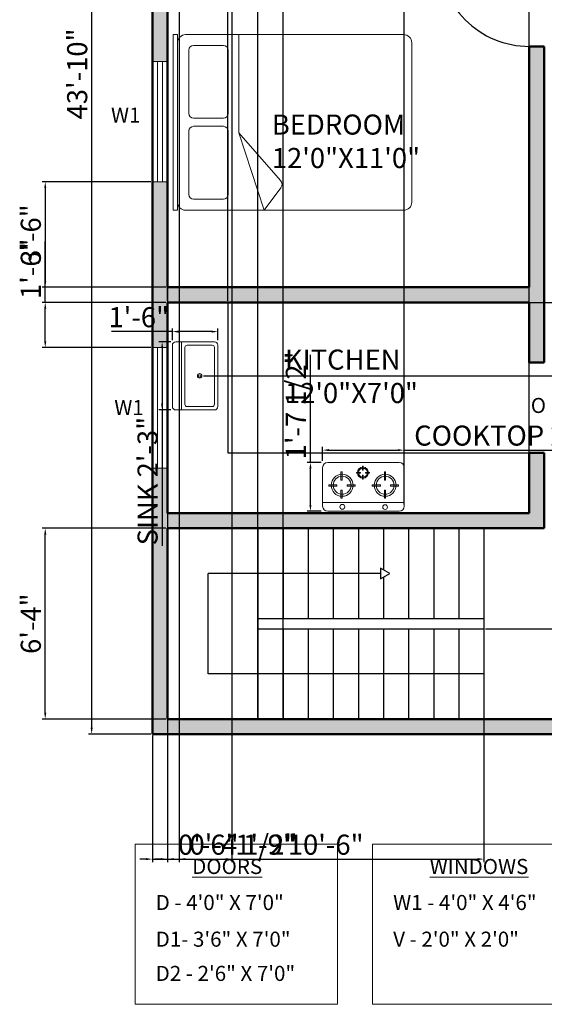
# Model space of a CAD drawing. Units: inches. Extents: x 3655 to 4051, y 2160 to 2854.
# Tile 1 of 3: x 3655 to 3863, y 2160 to 2552. Entities that reach past the tile are written whole.
import ezdxf

# ---------------------------------------------------------------- set-up
doc = ezdxf.new("R2010")
doc.units = ezdxf.units.IN
for name, color, linetype, lineweight in [('A-ANNO-DIMS', 2, 'Continuous', 18), ('A-ANNO-SCHD', 7, 'Continuous', 18), ('A-ANNO-TEXT', 7, 'Continuous', 18), ('A-AREA-IDEN', 7, 'Continuous', 25), ('A-DOOR', 3, 'Continuous', 25), ('A-EQPM', 9, 'Continuous', 18), ('A-FLOR-CASE', 8, 'Continuous', 25), ('A-FLOR-FIXT', 9, 'Continuous', 18), ('A-FLOR-STRS', 7, 'Continuous', 25), ('A-FURN', 8, 'Continuous', 18), ('A-GLAZ', 4, 'Continuous', 18), ('A-WALL', 7, 'Continuous', 50)]:
    doc.layers.add(name, color=color, linetype=linetype, lineweight=lineweight)
doc.layers.add('A-WALL-PATT', color=244, linetype='Continuous', lineweight=13, true_color=0x991b1e)
doc.styles.add('ATTR', font='romans.shx', dxfattribs={"width": 0.8, "height": 1.075})
doc.styles.get("Standard").update_dxf_attribs({"font": 'arial.ttf'})
doc.dimstyles.new('ISO-25', dxfattribs={"dimtxt": 8, "dimasz": 2.5, "dimexe": 1.25, "dimexo": 0.625, "dimtad": 1, "dimdec": 1, "dimlunit": 3, "dimtxsty": 'Standard', "dimcen": 2.5, "dimadec": 0, "dimazin": 0, "dimtfac": 1, "dimtdec": 1, "dimtmove": 0, "dimatfit": 3, "dimfxl": 1, "dimarcsym": 0})

# ---------------------------------------------------------------- blocks, each defined once
blk = doc.blocks.new('*U4')
for p, q in [((0, 0), (0, 6)), ((36, 0), (36, 6))]:
    blk.add_line(p, q)
blk.add_lwpolyline([(0, 0), (0, -36), (1.75, -36), (1.75, 0)], close=True)
blk.add_arc((0, 0), 36, 270, 0)
blk = doc.blocks.new('A$C164346CA')
for p, q in [((0, 2.035), (0, 2)), ((1.5, 2.035), (0, 2.035)), ((1.5, 2), (1.5, 2.035)), ((1.5, 2), (0, 2)), ((0, 1.93), (0, 0.07)), ((0.0919, 1.8624), (0.0919, 1.6069)), ((0.6731, 1.9024), (0.1319, 1.9024)), ((0.7131, 1.6069), (0.7131, 1.8624)), ((0.7828, 1.8624), (0.7828, 1.6069)), ((1.364, 1.9024), (0.8228, 1.9024)), ((1.404, 1.6069), (1.404, 1.8624)), ((1.5, 0.07), (1.5, 1.93)), ((0.1319, 1.5669), (0.6731, 1.5669)), ((0.8228, 1.5669), (1.364, 1.5669)), ((0.8395, 1.4761), (0, 1.4761)), ((0.8395, 1.4761), (1.2448, 1.12)), ((1.5, 1.2611), (0.8395, 1.4761)), ((1.3077, 1.1175), (1.5, 1.2611)), ((0.07, 0), (1.43, 0))]:
    blk.add_line(p, q)
for centre, radius, start, end in [((0.07, 1.93), 0.07, 90, 180), ((1.43, 1.93), 0.07, 0, 90), ((0.1319, 1.8624), 0.04, 90, 180), ((0.6731, 1.8624), 0.04, 0, 90), ((0.8228, 1.8624), 0.04, 90, 180), ((1.364, 1.8624), 0.04, 0, 90), ((0.1319, 1.6069), 0.04, 180, 270), ((0.6731, 1.6069), 0.04, 270, 0), ((0.8228, 1.6069), 0.04, 180, 270), ((1.364, 1.6069), 0.04, 270, 0), ((1.2778, 1.1575), 0.05, 228.69584, 306.75789), ((0.07, 0.07), 0.07, 180, 270), ((1.43, 0.07), 0.07, 270, 0)]:
    blk.add_arc(centre, radius, start, end)
blk = doc.blocks.new('A$C2A3C6842')
for p, q in [((0, 45), (0, 387)), ((45, 432), (675, 432)), ((351.6, 363.3), (351.6, 398.9)), ((351.6, 398.9), (357.3, 398.9)), ((357.3, 363.3), (351.6, 363.3)), ((357.3, 398.9), (357.3, 363.3)), ((720, 387), (720, 45)), ((161.8, 346.9), (173.2, 346.9)), ((161.8, 275.6), (161.8, 346.9)), ((173.2, 275.6), (161.8, 275.6)), ((173.2, 346.9), (173.2, 275.6)), ((298.4, 341.9), (298.4, 336.2)), ((334, 341.9), (298.4, 341.9)), ((298.4, 336.2), (334, 336.2)), ((334, 336.2), (334, 341.9)), ((357.3, 318.8), (351.6, 318.8)), ((351.6, 318.8), (351.6, 283.1)), ((351.6, 283.1), (357.3, 283.1)), ((357.3, 283.1), (357.3, 318.8)), ((378.5, 336.2), (378.5, 341.9)), ((378.5, 341.9), (414.2, 341.9)), ((414.2, 336.2), (378.5, 336.2)), ((414.2, 341.9), (414.2, 336.2)), ((544.7, 346.9), (556.1, 346.9)), ((544.7, 275.6), (544.7, 346.9)), ((556.1, 275.6), (544.7, 275.6)), ((556.1, 346.9), (556.1, 275.6)), ((55.3, 232.9), (55.3, 221.5)), ((126.6, 232.9), (55.3, 232.9)), ((55.3, 221.5), (126.6, 221.5)), ((126.6, 221.5), (126.6, 232.9)), ((173.2, 186.6), (161.8, 186.6)), ((161.8, 186.6), (161.8, 115.3)), ((173.2, 115.3), (173.2, 186.6)), ((215.6, 221.5), (215.6, 232.9)), ((215.6, 232.9), (286.9, 232.9)), ((286.9, 221.5), (215.6, 221.5)), ((286.9, 232.9), (286.9, 221.5)), ((438.2, 232.9), (438.2, 221.5)), ((509.5, 232.9), (438.2, 232.9)), ((438.2, 221.5), (509.5, 221.5)), ((509.5, 221.5), (509.5, 232.9)), ((556.1, 186.6), (544.7, 186.6)), ((544.7, 186.6), (544.7, 115.3)), ((556.1, 115.3), (556.1, 186.6)), ((598.5, 232.9), (669.8, 232.9)), ((598.5, 221.5), (598.5, 232.9)), ((669.8, 221.5), (598.5, 221.5)), ((669.8, 232.9), (669.8, 221.5)), ((161.8, 115.3), (173.2, 115.3)), ((544.7, 115.3), (556.1, 115.3)), ((1.2, 76.7), (719.9, 76.7)), ((675, 0), (45, 0))]:
    blk.add_line(p, q)
at = {"extrusion": (0, -1e-16, -1)}
for centre, major_axis, start_param, end_param in [((45, 387), (31.8, 31.8), 3.926991, 5.497787), ((172.2, 229.8), (-97.3, 0.1), -0.001099, 6.282086), ((551.8, 229.8), (-97.3, 0.1), -0.001099, 6.282086), ((173.7, 39), (-14.8, 14.8), 5.497787, 11.780972)]:
    blk.add_ellipse(centre, major_axis=major_axis, ratio=1, start_param=start_param, end_param=end_param, dxfattribs=at)
at = {"extrusion": (-1e-16, -1e-16, -1)}
blk.add_ellipse((355.1, 340.4), major_axis=(48.7, 0.1), ratio=1, start_param=3.144125, end_param=9.42731, dxfattribs=at)
at = {"extrusion": (-1e-16, 0, -1)}
for centre, major_axis, start_param, end_param in [((355.1, 340.4), (-39.7, 0), -0.000334, 6.282851), ((45, 45), (-31.8, 31.8), 3.926991, 5.497787)]:
    blk.add_ellipse(centre, major_axis=major_axis, ratio=1, start_param=start_param, end_param=end_param, dxfattribs=at)
at = {"extrusion": (0, 1e-16, -1)}
blk.add_ellipse((675, 387), major_axis=(-31.8, 31.8), ratio=1, start_param=0.785398, end_param=2.356194, dxfattribs=at)
at = {"extrusion": (-1e-16, -4e-16, -1)}
for centre in [(172.2, 229.8), (551.8, 229.8)]:
    blk.add_ellipse(centre, major_axis=(-79.3, 0), ratio=1, start_param=-0.0002116186602152, end_param=6.282973688519371, dxfattribs=at)
at = {"extrusion": (2e-16, -2e-16, -1)}
blk.add_ellipse((551.4, 36.4), major_axis=(14.8, 14.8), ratio=1, start_param=3.926991, end_param=10.210176, dxfattribs=at)
at = {"extrusion": (-2e-16, 1e-16, -1)}
blk.add_ellipse((675, 45), major_axis=(31.8, 31.8), ratio=1, start_param=0.785398, end_param=2.356194, dxfattribs=at)
at = {"text_generation_flag": 4, "flags": 9}
for tag in ['XSIZE', 'YSIZE']:
    blk.add_attdef(tag, (361.3, 264.9), '', height=0.45, rotation=180, dxfattribs=at)
blk = doc.blocks.new("30'' Sink Single PV")
blk.add_line((-15, -3.999996), (15, -3.999996))
for points in [[(-13.5, 0), (13.5, 0)], [(-15, -18.499996), (-15, -1.5)], [(15, -1.5), (15, -18.499996)], [(-13.5, -17.499996), (-13.5, -6.499996)], [(-12.5, -5.499996), (12.5, -5.499996)], [(13.5, -6.499996), (13.5, -17.499996)], [(13.5, -19.999996), (-13.5, -19.999996)], [(12.5, -18.499996), (-12.5, -18.499996)]]:
    blk.add_lwpolyline(points)
for radius in [1, 0.5]:
    blk.add_circle((0, -11.999996), radius)
for centre, radius, start, end in [((-13.5, -1.5), 1.5, 90, 180), ((13.5, -1.5), 1.5, 0, 90), ((-12.5, -6.499996), 1, 90, 180), ((12.5, -6.499996), 1, 0, 90), ((-13.5, -18.499996), 1.5, 180, 270), ((-12.5, -17.499996), 1, 180, 270), ((12.5, -17.499996), 1, 270, 0), ((13.5, -18.499996), 1.5, 270, 0)]:
    blk.add_arc(centre, radius, start, end)
at = {"style": 'ATTR', "width": 0.8, "flags": 9}
blk.add_attdef('ESTCODE', (0, 0), '', height=0.006, dxfattribs=at)
blk = doc.blocks.new('*D13')
at = {"layer": 'A-ANNO-DIMS', "color": 0, "lineweight": -2, "transparency": 16777216}
for p, q in [((3706.78, 2793.69), (3682, 2793.69)), ((3683.25, 2791.19), (3683.25, 2270.19)), ((3706.78, 2267.69), (3682, 2267.69))]:
    blk.add_line(p, q, dxfattribs=at)
at = {"layer": 'A-ANNO-DIMS', "color": 0, "transparency": 16777216}
for points in [[(3682.83, 2791.19), (3683.66, 2791.19), (3683.25, 2793.69)], [(3682.83, 2270.19), (3683.66, 2270.19), (3683.25, 2267.69)]]:
    blk.add_solid(points, dxfattribs=at)
at = {"layer": 'Defpoints', "color": 0, "transparency": 16777216}
for p in [(3707.41, 2793.69), (3683.25, 2267.69), (3707.41, 2267.69)]:
    blk.add_point(p, dxfattribs=at)
at = {"layer": 'A-ANNO-DIMS', "color": 0, "transparency": 16777216, "insert": (3678.53, 2530.69), "char_height": 8, "attachment_point": 5, "rotation": 90}
blk.add_mtext('43\'-10"', dxfattribs=at)
blk = doc.blocks.new('WIN-W1-48IN')
for p, q in [((0, 0), (0, 6)), ((48, 4), (0, 4)), ((48, 0), (48, 6)), ((48, 2), (0, 2))]:
    blk.add_line(p, q)
blk = doc.blocks.new('*D20')
at = {"layer": 'A-ANNO-DIMS', "color": 0, "lineweight": -2, "transparency": 16777216}
for p, q in [((3775.19, 2376.57), (3775.19, 2382.07)), ((3807.66, 2376.57), (3807.66, 2382.07)), ((3777.69, 2380.82), (3805.16, 2380.82)), ((3807.66, 2380.82), (3910.22, 2380.82))]:
    blk.add_line(p, q, dxfattribs=at)
at = {"layer": 'A-ANNO-DIMS', "color": 0, "transparency": 16777216}
for points in [[(3777.69, 2381.24), (3777.69, 2380.4), (3775.19, 2380.82)], [(3805.16, 2381.24), (3805.16, 2380.4), (3807.66, 2380.82)]]:
    blk.add_solid(points, dxfattribs=at)
at = {"layer": 'Defpoints', "color": 0, "transparency": 16777216}
for p in [(3807.66, 2380.82), (3775.19, 2375.95), (3807.66, 2375.95)]:
    blk.add_point(p, dxfattribs=at)
at = {"layer": 'A-ANNO-DIMS', "color": 0, "transparency": 16777216, "insert": (3860.19, 2385.58), "char_height": 8, "attachment_point": 5}
blk.add_mtext('COOKTOP 2\'-8 1/2"', dxfattribs=at)
blk = doc.blocks.new('*D21')
at = {"layer": 'A-ANNO-DIMS', "color": 0, "lineweight": -2, "transparency": 16777216}
for p, q in [((3770.32, 2375.95), (3770.32, 2418.85)), ((3774.57, 2375.95), (3769.07, 2375.95)), ((3770.32, 2358.97), (3770.32, 2373.45)), ((3774.57, 2356.47), (3769.07, 2356.47))]:
    blk.add_line(p, q, dxfattribs=at)
at = {"layer": 'A-ANNO-DIMS', "color": 0, "transparency": 16777216}
for points in [[(3769.91, 2373.45), (3770.74, 2373.45), (3770.32, 2375.95)], [(3769.91, 2358.97), (3770.74, 2358.97), (3770.32, 2356.47)]]:
    blk.add_solid(points, dxfattribs=at)
at = {"layer": 'Defpoints', "color": 0, "transparency": 16777216}
for p in [(3770.32, 2375.95), (3775.19, 2375.95), (3775.19, 2356.47)]:
    blk.add_point(p, dxfattribs=at)
at = {"layer": 'A-ANNO-DIMS', "color": 0, "transparency": 16777216, "insert": (3765.56, 2398.65), "char_height": 8, "attachment_point": 5, "rotation": 90}
blk.add_mtext('1\'-7 1/2"', dxfattribs=at)
blk = doc.blocks.new('*D22')
at = {"layer": 'A-ANNO-DIMS', "color": 0, "lineweight": -2, "transparency": 16777216}
for p, q in [((3879.35, 2535.27), (3879.35, 2656.5)), ((3895.99, 2535.27), (3878.1, 2535.27)), ((3879.35, 2422.65), (3879.35, 2532.77)), ((3895.99, 2420.15), (3878.1, 2420.15))]:
    blk.add_line(p, q, dxfattribs=at)
at = {"layer": 'A-ANNO-DIMS', "color": 0, "transparency": 16777216}
for points in [[(3878.93, 2532.77), (3879.76, 2532.77), (3879.35, 2535.27)], [(3878.93, 2422.65), (3879.76, 2422.65), (3879.35, 2420.15)]]:
    blk.add_solid(points, dxfattribs=at)
at = {"layer": 'Defpoints', "color": 0, "transparency": 16777216}
for p in [(3879.35, 2535.27), (3896.61, 2535.27), (3896.61, 2420.15)]:
    blk.add_point(p, dxfattribs=at)
at = {"layer": 'A-ANNO-DIMS', "color": 0, "transparency": 16777216, "insert": (3874.58, 2597.13), "char_height": 8, "attachment_point": 5, "rotation": 90}
blk.add_mtext('SEATING GROUP 9\'-7"', dxfattribs=at)
blk = doc.blocks.new('*D24')
at = {"layer": 'A-ANNO-DIMS', "color": 0, "lineweight": -2, "transparency": 16777216}
for p, q in [((3714.75, 2423.96), (3710.05, 2423.96)), ((3711.3, 2421.46), (3711.3, 2399.31)), ((3714.75, 2396.81), (3710.05, 2396.81)), ((3711.3, 2396.81), (3711.3, 2342.65))]:
    blk.add_line(p, q, dxfattribs=at)
at = {"layer": 'A-ANNO-DIMS', "color": 0, "transparency": 16777216}
for points in [[(3710.88, 2421.46), (3711.72, 2421.46), (3711.3, 2423.96)], [(3710.88, 2399.31), (3711.72, 2399.31), (3711.3, 2396.81)]]:
    blk.add_solid(points, dxfattribs=at)
at = {"layer": 'Defpoints', "color": 0, "transparency": 16777216}
for p in [(3715.37, 2423.96), (3711.3, 2396.81), (3715.37, 2396.81)]:
    blk.add_point(p, dxfattribs=at)
at = {"layer": 'A-ANNO-DIMS', "color": 0, "transparency": 16777216, "insert": (3706.54, 2368.48), "char_height": 8, "attachment_point": 5, "rotation": 90}
blk.add_mtext('SINK 2\'-3"', dxfattribs=at)
blk = doc.blocks.new('*D25')
at = {"layer": 'A-ANNO-DIMS', "color": 0, "lineweight": -2, "transparency": 16777216}
for p, q in [((3715.37, 2424.59), (3715.37, 2429.29)), ((3733.48, 2424.59), (3733.48, 2429.29)), ((3715.37, 2428.04), (3691.11, 2428.04)), ((3730.98, 2428.04), (3717.87, 2428.04))]:
    blk.add_line(p, q, dxfattribs=at)
at = {"layer": 'A-ANNO-DIMS', "color": 0, "transparency": 16777216}
for points in [[(3717.87, 2428.45), (3717.87, 2427.62), (3715.37, 2428.04)], [(3730.98, 2428.45), (3730.98, 2427.62), (3733.48, 2428.04)]]:
    blk.add_solid(points, dxfattribs=at)
at = {"layer": 'Defpoints', "color": 0, "transparency": 16777216}
for p in [(3715.37, 2428.04), (3715.37, 2423.96), (3733.48, 2423.96)]:
    blk.add_point(p, dxfattribs=at)
at = {"layer": 'A-ANNO-DIMS', "color": 0, "transparency": 16777216, "insert": (3701.99, 2432.75), "char_height": 8, "attachment_point": 5}
blk.add_mtext('1\'-6"', dxfattribs=at)
blk = doc.blocks.new('*D29')
at = {"layer": 'A-ANNO-DIMS', "color": 0, "lineweight": -2, "transparency": 16777216}
for p, q in [((3713.41, 2273.07), (3713.41, 2216.63)), ((3839.41, 2273.07), (3839.41, 2216.63)), ((3715.91, 2217.88), (3836.91, 2217.88))]:
    blk.add_line(p, q, dxfattribs=at)
at = {"layer": 'A-ANNO-DIMS', "color": 0, "transparency": 16777216}
for points in [[(3715.91, 2218.3), (3715.91, 2217.47), (3713.41, 2217.88)], [(3836.91, 2218.3), (3836.91, 2217.47), (3839.41, 2217.88)]]:
    blk.add_solid(points, dxfattribs=at)
at = {"layer": 'Defpoints', "color": 0, "transparency": 16777216}
for p in [(3713.41, 2273.69), (3839.41, 2273.69), (3839.41, 2217.88)]:
    blk.add_point(p, dxfattribs=at)
at = {"layer": 'A-ANNO-DIMS', "color": 0, "transparency": 16777216, "insert": (3776.41, 2222.59), "char_height": 8, "attachment_point": 5}
blk.add_mtext('10\'-6"', dxfattribs=at)
blk = doc.blocks.new('*D30')
at = {"layer": 'A-ANNO-DIMS', "color": 0, "lineweight": -2, "transparency": 16777216}
for p, q in [((3712.78, 2349.69), (3663.52, 2349.69)), ((3664.77, 2276.19), (3664.77, 2347.19)), ((3712.78, 2273.69), (3663.52, 2273.69))]:
    blk.add_line(p, q, dxfattribs=at)
at = {"layer": 'A-ANNO-DIMS', "color": 0, "transparency": 16777216}
for points in [[(3664.36, 2347.19), (3665.19, 2347.19), (3664.77, 2349.69)], [(3664.36, 2276.19), (3665.19, 2276.19), (3664.77, 2273.69)]]:
    blk.add_solid(points, dxfattribs=at)
at = {"layer": 'Defpoints', "color": 0, "transparency": 16777216}
for p in [(3664.77, 2349.69), (3713.41, 2349.69), (3713.41, 2273.69)]:
    blk.add_point(p, dxfattribs=at)
at = {"layer": 'A-ANNO-DIMS', "color": 0, "transparency": 16777216, "insert": (3660.06, 2311.69), "char_height": 8, "attachment_point": 5, "rotation": 90}
blk.add_mtext('6\'-4"', dxfattribs=at)
blk = doc.blocks.new('*D31')
at = {"layer": 'A-ANNO-DIMS', "color": 0, "lineweight": -2, "transparency": 16777216}
for p, q in [((3713.41, 2440.32), (3713.41, 2825.74)), ((3734.91, 2824.49), (3715.91, 2824.49)), ((3737.41, 2440.32), (3737.41, 2825.74))]:
    blk.add_line(p, q, dxfattribs=at)
at = {"layer": 'A-ANNO-DIMS', "color": 0, "transparency": 16777216}
for points in [[(3715.91, 2824.91), (3715.91, 2824.07), (3713.41, 2824.49)], [(3734.91, 2824.91), (3734.91, 2824.07), (3737.41, 2824.49)]]:
    blk.add_solid(points, dxfattribs=at)
at = {"layer": 'Defpoints', "color": 0, "transparency": 16777216}
for p in [(3713.41, 2824.49), (3713.41, 2439.69), (3737.41, 2439.69)]:
    blk.add_point(p, dxfattribs=at)
at = {"layer": 'A-ANNO-DIMS', "color": 0, "transparency": 16777216, "insert": (3725.41, 2829.2), "char_height": 8, "attachment_point": 5}
blk.add_mtext('2\'-0"', dxfattribs=at)
blk = doc.blocks.new('*D38')
at = {"layer": 'A-ANNO-DIMS', "color": 0, "lineweight": -2, "transparency": 16777216}
for p, q in [((3713.41, 2273.07), (3713.41, 2216.63)), ((3707.41, 2267.07), (3707.41, 2216.63)), ((3704.91, 2217.88), (3702.41, 2217.88)), ((3707.41, 2217.88), (3713.41, 2217.88)), ((3715.91, 2217.88), (3740.93, 2217.88))]:
    blk.add_line(p, q, dxfattribs=at)
at = {"layer": 'A-ANNO-DIMS', "color": 0, "transparency": 16777216}
for points in [[(3704.91, 2218.3), (3704.91, 2217.47), (3707.41, 2217.88)], [(3715.91, 2218.3), (3715.91, 2217.47), (3713.41, 2217.88)]]:
    blk.add_solid(points, dxfattribs=at)
at = {"layer": 'Defpoints', "color": 0, "transparency": 16777216}
for p in [(3713.41, 2273.69), (3707.41, 2267.69), (3713.41, 2217.88)]:
    blk.add_point(p, dxfattribs=at)
at = {"layer": 'A-ANNO-DIMS', "color": 0, "transparency": 16777216, "insert": (3729.67, 2222.59), "char_height": 8, "attachment_point": 5}
blk.add_mtext('0\'-6"', dxfattribs=at)
blk = doc.blocks.new('*D39')
at = {"layer": 'A-ANNO-DIMS', "color": 0, "lineweight": -2, "transparency": 16777216}
for p, q in [((3664.77, 2439.69), (3664.77, 2463.95)), ((3712.78, 2439.69), (3663.52, 2439.69)), ((3664.77, 2424.19), (3664.77, 2437.19)), ((3706.78, 2421.69), (3663.52, 2421.69))]:
    blk.add_line(p, q, dxfattribs=at)
at = {"layer": 'A-ANNO-DIMS', "color": 0, "transparency": 16777216}
for points in [[(3664.36, 2437.19), (3665.19, 2437.19), (3664.77, 2439.69)], [(3664.36, 2424.19), (3665.19, 2424.19), (3664.77, 2421.69)]]:
    blk.add_solid(points, dxfattribs=at)
at = {"layer": 'Defpoints', "color": 0, "transparency": 16777216}
for p in [(3664.77, 2439.69), (3713.41, 2439.69), (3707.41, 2421.69)]:
    blk.add_point(p, dxfattribs=at)
at = {"layer": 'A-ANNO-DIMS', "color": 0, "transparency": 16777216, "insert": (3660.06, 2453.07), "char_height": 8, "attachment_point": 5, "rotation": 90}
blk.add_mtext('1\'-6"', dxfattribs=at)
blk = doc.blocks.new('*D40')
at = {"layer": 'A-ANNO-DIMS', "color": 0, "lineweight": -2, "transparency": 16777216}
for p, q in [((3706.78, 2487.69), (3663.52, 2487.69)), ((3664.77, 2485.19), (3664.77, 2448.19)), ((3712.78, 2445.69), (3663.52, 2445.69))]:
    blk.add_line(p, q, dxfattribs=at)
at = {"layer": 'A-ANNO-DIMS', "color": 0, "transparency": 16777216}
for points in [[(3664.36, 2485.19), (3665.19, 2485.19), (3664.77, 2487.69)], [(3664.36, 2448.19), (3665.19, 2448.19), (3664.77, 2445.69)]]:
    blk.add_solid(points, dxfattribs=at)
at = {"layer": 'Defpoints', "color": 0, "transparency": 16777216}
for p in [(3707.41, 2487.69), (3664.77, 2445.69), (3713.41, 2445.69)]:
    blk.add_point(p, dxfattribs=at)
at = {"layer": 'A-ANNO-DIMS', "color": 0, "transparency": 16777216, "insert": (3660.06, 2466.69), "char_height": 8, "attachment_point": 5, "rotation": 90}
blk.add_mtext('3\'-6"', dxfattribs=at)
blk = doc.blocks.new('*D45')
at = {"layer": 'A-ANNO-DIMS', "color": 0, "lineweight": -2, "transparency": 16777216}
for p, q in [((3749.41, 2274.32), (3749.41, 2825.74)), ((3751.91, 2824.49), (3756.91, 2824.49)), ((3759.41, 2274.32), (3759.41, 2825.74)), ((3759.41, 2824.49), (3790.64, 2824.49))]:
    blk.add_line(p, q, dxfattribs=at)
at = {"layer": 'A-ANNO-DIMS', "color": 0, "transparency": 16777216}
for points in [[(3751.91, 2824.91), (3751.91, 2824.07), (3749.41, 2824.49)], [(3756.91, 2824.91), (3756.91, 2824.07), (3759.41, 2824.49)]]:
    blk.add_solid(points, dxfattribs=at)
at = {"layer": 'Defpoints', "color": 0, "transparency": 16777216}
for p in [(3759.41, 2824.49), (3749.41, 2273.69), (3759.41, 2273.69)]:
    blk.add_point(p, dxfattribs=at)
at = {"layer": 'A-ANNO-DIMS', "color": 0, "transparency": 16777216, "insert": (3776.28, 2829.2), "char_height": 8, "attachment_point": 5}
blk.add_mtext('0\'-10"', dxfattribs=at)
blk = doc.blocks.new('*D46')
at = {"layer": 'A-ANNO-DIMS', "color": 0, "lineweight": -2, "transparency": 16777216}
for p, q in [((3840.03, 2309.69), (4045.46, 2309.69)), ((4044.21, 2276.19), (4044.21, 2307.19)), ((3840.03, 2273.69), (4045.46, 2273.69))]:
    blk.add_line(p, q, dxfattribs=at)
at = {"layer": 'A-ANNO-DIMS', "color": 0, "transparency": 16777216}
for points in [[(4043.79, 2307.19), (4044.63, 2307.19), (4044.21, 2309.69)], [(4043.79, 2276.19), (4044.63, 2276.19), (4044.21, 2273.69)]]:
    blk.add_solid(points, dxfattribs=at)
at = {"layer": 'Defpoints', "color": 0, "transparency": 16777216}
for p in [(3839.41, 2309.69), (4044.21, 2309.69), (3839.41, 2273.69)]:
    blk.add_point(p, dxfattribs=at)
at = {"layer": 'A-ANNO-DIMS', "color": 0, "transparency": 16777216, "insert": (4039.5, 2291.69), "char_height": 8, "attachment_point": 5, "rotation": 90}
blk.add_mtext('3\'-0"', dxfattribs=at)
blk = doc.blocks.new('*D48')
at = {"layer": 'A-ANNO-DIMS', "color": 0, "lineweight": -2, "transparency": 16777216}
for p, q in [((3718.07, 2593.79), (3718.07, 2216.63)), ((3739.07, 2593.79), (3739.07, 2216.63)), ((3720.57, 2217.88), (3736.57, 2217.88)), ((3739.07, 2217.88), (3763.34, 2217.88))]:
    blk.add_line(p, q, dxfattribs=at)
at = {"layer": 'A-ANNO-DIMS', "color": 0, "transparency": 16777216}
for points in [[(3720.57, 2218.3), (3720.57, 2217.47), (3718.07, 2217.88)], [(3736.57, 2218.3), (3736.57, 2217.47), (3739.07, 2217.88)]]:
    blk.add_solid(points, dxfattribs=at)
at = {"layer": 'Defpoints', "color": 0, "transparency": 16777216}
for p in [(3718.07, 2594.42), (3739.07, 2594.42), (3739.07, 2217.88)]:
    blk.add_point(p, dxfattribs=at)
at = {"layer": 'A-ANNO-DIMS', "color": 0, "transparency": 16777216, "insert": (3752.46, 2222.59), "char_height": 8, "attachment_point": 5}
blk.add_mtext('1\'-9"', dxfattribs=at)
blk = doc.blocks.new('*D50')
at = {"layer": 'A-ANNO-DIMS', "color": 0, "lineweight": -2, "transparency": 16777216}
for p, q in [((3718.07, 2585.79), (3718.07, 2216.63)), ((3713.41, 2583.07), (3713.41, 2216.63)), ((3710.91, 2217.88), (3708.41, 2217.88)), ((3713.41, 2217.88), (3718.07, 2217.88)), ((3720.57, 2217.88), (3764.23, 2217.88))]:
    blk.add_line(p, q, dxfattribs=at)
at = {"layer": 'A-ANNO-DIMS', "color": 0, "transparency": 16777216}
for points in [[(3710.91, 2218.3), (3710.91, 2217.47), (3713.41, 2217.88)], [(3720.57, 2218.3), (3720.57, 2217.47), (3718.07, 2217.88)]]:
    blk.add_solid(points, dxfattribs=at)
at = {"layer": 'Defpoints', "color": 0, "transparency": 16777216}
for p in [(3718.07, 2586.42), (3713.41, 2583.69), (3718.07, 2217.88)]:
    blk.add_point(p, dxfattribs=at)
at = {"layer": 'A-ANNO-DIMS', "color": 0, "transparency": 16777216, "insert": (3743.65, 2222.64), "char_height": 8, "attachment_point": 5}
blk.add_mtext('0\'-4 1/2"', dxfattribs=at)
blk = doc.blocks.new('*D51')
at = {"layer": 'A-ANNO-DIMS', "color": 0, "lineweight": -2, "transparency": 16777216}
for p, q in [((4044.21, 2588.92), (4044.21, 2591.42)), ((3739.7, 2586.42), (4045.46, 2586.42)), ((4044.21, 2586.42), (4044.21, 2583.69)), ((3798.03, 2583.69), (4045.46, 2583.69)), ((4044.21, 2581.19), (4044.21, 2537.53))]:
    blk.add_line(p, q, dxfattribs=at)
at = {"layer": 'A-ANNO-DIMS', "color": 0, "transparency": 16777216}
for points in [[(4043.79, 2588.92), (4044.63, 2588.92), (4044.21, 2586.42)], [(4043.79, 2581.19), (4044.63, 2581.19), (4044.21, 2583.69)]]:
    blk.add_solid(points, dxfattribs=at)
at = {"layer": 'Defpoints', "color": 0, "transparency": 16777216}
for p in [(3739.07, 2586.42), (3797.41, 2583.69), (4044.21, 2583.69)]:
    blk.add_point(p, dxfattribs=at)
at = {"layer": 'A-ANNO-DIMS', "color": 0, "transparency": 16777216, "insert": (4039.45, 2558.11), "char_height": 8, "attachment_point": 5, "rotation": 90}
blk.add_mtext('0\'-2 1/2"', dxfattribs=at)
blk = doc.blocks.new('*D52')
at = {"layer": 'A-ANNO-DIMS', "color": 0, "lineweight": -2, "transparency": 16777216}
for p, q in [((3807.66, 2359.12), (3807.66, 2825.74)), ((3810.16, 2824.49), (3854.91, 2824.49)), ((3857.41, 2356.32), (3857.41, 2825.74))]:
    blk.add_line(p, q, dxfattribs=at)
at = {"layer": 'A-ANNO-DIMS', "color": 0, "transparency": 16777216}
for points in [[(3810.16, 2824.91), (3810.16, 2824.07), (3807.66, 2824.49)], [(3854.91, 2824.91), (3854.91, 2824.07), (3857.41, 2824.49)]]:
    blk.add_solid(points, dxfattribs=at)
at = {"layer": 'Defpoints', "color": 0, "transparency": 16777216}
for p in [(3857.41, 2824.49), (3807.66, 2358.5), (3857.41, 2355.69)]:
    blk.add_point(p, dxfattribs=at)
at = {"layer": 'A-ANNO-DIMS', "color": 0, "transparency": 16777216, "insert": (3832.54, 2829.25), "char_height": 8, "attachment_point": 5}
blk.add_mtext('4\'-1 1/2"', dxfattribs=at)
blk = doc.blocks.new('*D53')
at = {"layer": 'A-ANNO-DIMS', "color": 0, "lineweight": -2, "transparency": 16777216}
for p, q in [((4044.21, 2439.69), (4044.21, 2483.48)), ((3738.03, 2439.69), (4045.46, 2439.69)), ((4044.21, 2412.89), (4044.21, 2437.19)), ((3727.77, 2410.39), (4045.46, 2410.39))]:
    blk.add_line(p, q, dxfattribs=at)
at = {"layer": 'A-ANNO-DIMS', "color": 0, "transparency": 16777216}
for points in [[(4043.79, 2437.19), (4044.63, 2437.19), (4044.21, 2439.69)], [(4043.79, 2412.89), (4044.63, 2412.89), (4044.21, 2410.39)]]:
    blk.add_solid(points, dxfattribs=at)
at = {"layer": 'Defpoints', "color": 0, "transparency": 16777216}
for p in [(3737.41, 2439.69), (4044.21, 2439.69), (3727.14, 2410.39)]:
    blk.add_point(p, dxfattribs=at)
at = {"layer": 'A-ANNO-DIMS', "color": 0, "transparency": 16777216, "insert": (4039.45, 2462.84), "char_height": 8, "attachment_point": 5, "rotation": 90}
blk.add_mtext('2\'-5 1/2"', dxfattribs=at)

msp = doc.modelspace()

# ---------------------------------------------------------------- hatches: boundary and pattern name
at = {"layer": 'A-WALL-PATT'}
h = msp.add_hatch(color=256, dxfattribs=at)
h.dxf.hatch_style = 1
h.paths.add_polyline_path([(3713.41, 2787.69), (3761.41, 2787.69), (3761.41, 2793.69), (3707.41, 2793.69), (3707.41, 2622.69), (3713.41, 2622.69), (3713.41, 2637.69), (3821.41, 2637.69), (3821.41, 2643.69), (3713.41, 2643.69)])
h.paths.add_polyline_path([(3863.41, 2787.69), (3911.41, 2787.69), (3911.41, 2793.69), (3809.41, 2793.69), (3809.41, 2787.69), (3857.41, 2787.69), (3857.41, 2637.69), (3863.41, 2637.69)])
h.paths.add_polyline_path([(4013.41, 2793.69), (3959.41, 2793.69), (3959.41, 2787.69), (4007.41, 2787.69), (4007.41, 2643.69), (3899.41, 2643.69), (3899.41, 2637.69), (3917.41, 2637.69), (3917.41, 2577.69), (3947.41, 2577.69), (3947.41, 2583.69), (3923.41, 2583.69), (3923.41, 2637.69), (4007.41, 2637.69), (4007.41, 2583.69), (3983.41, 2583.69), (3983.41, 2577.69), (4007.41, 2577.69), (4007.41, 2500.75), (4013.41, 2500.75)])
h.paths.add_polyline_path([(3863.41, 2583.69), (3803.41, 2583.69), (3803.41, 2607.69), (3797.41, 2607.69), (3797.41, 2583.69), (3713.41, 2583.69), (3713.41, 2598.69), (3707.41, 2598.69), (3707.41, 2535.69), (3713.41, 2535.69), (3713.41, 2577.69), (3863.41, 2577.69)])
h.paths.add_polyline_path([(3863.41, 2541.69), (3857.41, 2541.69), (3857.41, 2445.69), (3713.41, 2445.69), (3713.41, 2487.69), (3707.41, 2487.69), (3707.41, 2421.69), (3713.41, 2421.69), (3713.41, 2439.69), (3857.41, 2439.69), (3857.41, 2415.69), (3863.41, 2415.69)])
h.paths.add_polyline_path([(3863.41, 2379.69), (3857.41, 2379.69), (3857.41, 2355.69), (3713.41, 2355.69), (3713.41, 2373.69), (3707.41, 2373.69), (3707.41, 2267.69), (3907.77, 2267.69), (3907.77, 2273.69), (3713.41, 2273.69), (3713.41, 2349.69), (3863.41, 2349.69)])
h.paths.add_polyline_path([(3951.59, 2273.69), (3943.77, 2273.69), (3943.77, 2267.69), (3951.59, 2267.69)])
h.paths.add_polyline_path([(4013.41, 2452.75), (4007.41, 2452.75), (4007.41, 2273.69), (3999.59, 2273.69), (3999.59, 2267.69), (4013.41, 2267.69)])

# ---------------------------------------------------------------- linework, layer by layer
at = {"layer": 'A-ANNO-SCHD'}
for points in [[(3700.51, 2223.88), (3781.07, 2223.88), (3781.07, 2160.04), (3700.51, 2160.04)], [(3795.04, 2223.88), (3875.6, 2223.88), (3875.6, 2160.04), (3795.04, 2160.04)]]:
    msp.add_lwpolyline(points, close=True, dxfattribs=at)
at = {"layer": 'A-FLOR-CASE'}
for p, q in [((3737.41, 2439.69), (3737.41, 2379.69)), ((3737.41, 2379.69), (3857.41, 2379.69))]:
    msp.add_line(p, q, dxfattribs=at)
at = {"layer": 'A-FLOR-STRS'}
for p, q in [((3749.41, 2349.69), (3749.41, 2273.69)), ((3759.41, 2349.69), (3759.41, 2313.69)), ((3769.41, 2349.69), (3769.41, 2313.69)), ((3779.41, 2349.69), (3779.41, 2313.69)), ((3789.41, 2349.69), (3789.41, 2313.69)), ((3799.41, 2349.69), (3799.41, 2333.13)), ((3809.41, 2349.69), (3809.41, 2313.69)), ((3819.41, 2349.69), (3819.41, 2313.69)), ((3829.41, 2349.69), (3829.41, 2313.69)), ((3839.41, 2349.69), (3839.41, 2273.69)), ((3729.62, 2291.69), (3729.62, 2331.69)), ((3798.16, 2331.69), (3729.62, 2331.69)), ((3799.41, 2330.25), (3799.41, 2313.69)), ((3749.41, 2313.69), (3839.41, 2313.69)), ((3749.41, 2309.69), (3839.41, 2309.69)), ((3759.41, 2309.69), (3759.41, 2273.69)), ((3769.41, 2309.69), (3769.41, 2273.69)), ((3779.41, 2309.69), (3779.41, 2273.69)), ((3789.41, 2309.69), (3789.41, 2273.69)), ((3799.41, 2309.69), (3799.41, 2273.69)), ((3809.41, 2309.69), (3809.41, 2273.69)), ((3819.41, 2309.69), (3819.41, 2273.69)), ((3829.41, 2309.69), (3829.41, 2273.69)), ((3839.41, 2291.69), (3729.62, 2291.69))]:
    msp.add_line(p, q, dxfattribs=at)
msp.add_lwpolyline([(3801.9, 2331.69), (3798.16, 2333.85), (3798.16, 2329.53)], close=True, dxfattribs=at)
at = {"layer": 'A-WALL'}
for p, q in [((3707.41, 2793.69), (3707.41, 2267.69)), ((3713.41, 2577.69), (3713.41, 2445.69)), ((3857.41, 2541.69), (3857.41, 2445.69)), ((3857.41, 2541.69), (3863.41, 2541.69)), ((3863.41, 2541.69), (3863.41, 2415.69)), ((3713.41, 2445.69), (3857.41, 2445.69)), ((3713.41, 2439.69), (3857.41, 2439.69)), ((3713.41, 2439.69), (3713.41, 2355.69)), ((3857.41, 2439.69), (3857.41, 2415.69)), ((3857.41, 2415.69), (3863.41, 2415.69)), ((3857.41, 2379.69), (3863.41, 2379.69)), ((3857.41, 2379.69), (3857.41, 2355.69)), ((3863.41, 2379.69), (3863.41, 2349.69)), ((3713.41, 2355.69), (3857.41, 2355.69)), ((3713.41, 2349.69), (3863.41, 2349.69)), ((3713.41, 2349.69), (3713.41, 2273.69)), ((3713.41, 2273.69), (3907.77, 2273.69)), ((3707.41, 2267.69), (3907.77, 2267.69))]:
    msp.add_line(p, q, dxfattribs=at)

# ---------------------------------------------------------------- block references
at = {"layer": 'A-DOOR', "rotation": 270}
msp.add_blockref('*U4', (3857.41, 2577.69), dxfattribs=at)
at = {"layer": 'A-EQPM', "xscale": 0.0450941956703693, "yscale": 0.0450941956703693, "zscale": 0.0450941956703693}
msp.add_blockref('A$C2A3C6842', (3775.19, 2356.47), dxfattribs=at)
at = {"layer": 'A-FLOR-FIXT', "xscale": -0.904986321808974, "yscale": 0.904986321808974, "zscale": 0.904986321808974, "rotation": 90}
msp.add_blockref("30'' Sink Single PV", (3715.38, 2410.39), dxfattribs=at)
at = {"layer": 'A-FURN', "xscale": -46.65071231409348, "yscale": 46.65071231409348, "zscale": 46.65071231409348, "rotation": 90}
msp.add_blockref('A$C164346CA', (3810.68, 2546.35), dxfattribs=at)
at = {"layer": 'A-GLAZ', "rotation": 269.9999999999989}
for p in [(3707.41, 2535.69), (3707.41, 2421.69)]:
    msp.add_blockref('WIN-W1-48IN', p, dxfattribs=at)

# ---------------------------------------------------------------- texts
at = {"layer": 'A-ANNO-SCHD', "char_height": 6, "attachment_point": 1}
for s, width, insert in [('{\\LDOORS}', 13.8821, (3723.26, 2217.95)), ('{\\LWINDOWS}', 13.8821, (3817.79, 2217.95)), ('D - 4\'0" X 7\'0"', 70.1276, (3708.73, 2203.6)), ('W1 - 4\'0" X 4\'6"', 70.1276, (3803.26, 2203.6)), ('D1- 3\'6" X 7\'0"', 70.1276, (3708.73, 2188.98)), ('V - 2\'0" X 2\'0"', 70.1276, (3803.26, 2188.98)), ('D2 - 2\'6" X 7\'0"', 70.1276, (3708.73, 2175.35))]:
    msp.add_mtext_dynamic_manual_height_columns(s, width=width, gutter_width=12.5, heights=[0], dxfattribs=dict(at, insert=insert))
at = {"layer": 'A-ANNO-TEXT', "char_height": 6, "attachment_point": 1}
for s, insert in [('W1', (3690.94, 2517.3)), ('W1', (3692.26, 2400.79)), ('O', (3858.03, 2401.62))]:
    msp.add_mtext_dynamic_manual_height_columns(s, width=13.8821, gutter_width=12.5, heights=[0], dxfattribs=dict(at, insert=insert))
at = {"layer": 'A-AREA-IDEN', "char_height": 8, "attachment_point": 1}
for s, insert in [('BEDROOM\\P12\'0"X11\'0"', (3754.95, 2514.53)), ('KITCHEN\\P12\'0"X7\'0"', (3760.17, 2420.9))]:
    msp.add_mtext_dynamic_manual_height_columns(s, width=84.0989, gutter_width=12.5, heights=[0], dxfattribs=dict(at, insert=insert))

# ---------------------------------------------------------------- dimensions: what is measured, and where the dimension line sits
at = {"layer": 'A-ANNO-DIMS'}
for base, p1, p2, picture, middle in [((3857.4098, 2824.4907), (3807.6627, 2358.4982), (3857.4098, 2355.6907), '*D52', (3832.5363, 2829.2521)), ((3713.41, 2824.49), (3737.41, 2439.69), (3713.41, 2439.69), '*D31', (3725.41, 2829.2)), ((3759.41, 2824.49), (3749.41, 2273.69), (3759.41, 2273.69), '*D45', (3776.28, 2829.2)), ((3739.07, 2217.88), (3718.07, 2594.42), (3739.07, 2594.42), '*D48', (3752.46, 2222.59)), ((3718.07, 2217.88), (3713.41, 2583.69), (3718.07, 2586.42), '*D50', (3743.65, 2222.64)), ((3713.41, 2217.88), (3707.41, 2267.69), (3713.41, 2273.69), '*D38', (3729.67, 2222.59)), ((3839.41, 2217.88), (3713.41, 2273.69), (3839.41, 2273.69), '*D29', (3776.41, 2222.59))]:
    dim = msp.add_linear_dim(base=base, p1=p1, p2=p2, dimstyle='ISO-25', override={"dimdec": 1, "dimlfac": 1, "dimrnd": 0, "dimzin": 1, "dimdsep": 46, "dimlunit": 4, "dimfrac": 2}, dxfattribs=at)
    dim.commit()
    dim.dimension.update_dxf_attribs({"geometry": picture, "text_midpoint": middle})
for base, p1, p2, angle, override, picture, middle in [((3683.25, 2267.69), (3707.41, 2793.69), (3707.41, 2267.69), 90, {"dimclrd": 0, "dimclre": 0, "dimclrt": 0}, '*D13', (3678.53, 2530.69)), ((4044.21, 2583.69), (3739.07, 2586.42), (3797.41, 2583.69), 90, {"dimdec": 1, "dimlfac": 1, "dimrnd": 0, "dimzin": 1, "dimdsep": 46, "dimlunit": 4, "dimfrac": 2}, '*D51', (4039.45, 2558.11)), ((3664.77, 2445.69), (3707.41, 2487.69), (3713.41, 2445.69), 90, {"dimdec": 1, "dimlfac": 1, "dimrnd": 0, "dimzin": 1, "dimdsep": 46, "dimlunit": 4, "dimfrac": 2}, '*D40', (3660.06, 2466.69)), ((4044.21, 2439.69), (3727.14, 2410.39), (3737.41, 2439.69), 90, {"dimdec": 1, "dimlfac": 1, "dimrnd": 0, "dimzin": 1, "dimdsep": 46, "dimlunit": 4, "dimfrac": 2}, '*D53', (4039.45, 2462.84)), ((3664.77, 2439.69), (3707.41, 2421.69), (3713.41, 2439.69), 90, {"dimdec": 1, "dimlfac": 1, "dimrnd": 0, "dimzin": 1, "dimdsep": 46, "dimlunit": 4, "dimfrac": 2}, '*D39', (3660.06, 2453.07)), ((3715.37, 2428.04), (3733.48, 2423.96), (3715.37, 2423.96), 180, {"dimdec": 1, "dimlfac": 1, "dimrnd": 0, "dimzin": 1, "dimdsep": 46, "dimlunit": 4, "dimfrac": 2}, '*D25', (3701.99, 2432.75)), ((3770.32, 2375.95), (3775.19, 2356.47), (3775.19, 2375.95), 90, {"dimdec": 1, "dimlfac": 1, "dimrnd": 0, "dimzin": 1, "dimdsep": 46, "dimlunit": 4, "dimfrac": 2}, '*D21', (3765.56, 2398.65)), ((3664.77, 2349.69), (3713.41, 2273.69), (3713.41, 2349.69), 90, {"dimdec": 1, "dimlfac": 1, "dimrnd": 0, "dimzin": 1, "dimdsep": 46, "dimlunit": 4, "dimfrac": 2}, '*D30', (3660.06, 2311.69)), ((4044.21, 2309.69), (3839.41, 2273.69), (3839.41, 2309.69), 90, {"dimdec": 1, "dimlfac": 1, "dimrnd": 0, "dimzin": 1, "dimdsep": 46, "dimlunit": 4, "dimfrac": 2}, '*D46', (4039.5, 2291.69))]:
    dim = msp.add_linear_dim(base=base, p1=p1, p2=p2, angle=angle, dimstyle='ISO-25', override=override, dxfattribs=at)
    dim.commit()
    dim.dimension.update_dxf_attribs({"geometry": picture, "text_midpoint": middle})
for base, p1, p2, angle, text, picture, middle in [((3879.35, 2535.27), (3896.61, 2420.15), (3896.61, 2535.27), 90, 'SEATING GROUP <>', '*D22', (3874.58, 2597.13)), ((3711.2997, 2396.8139), (3715.3722, 2423.9635), (3715.3722, 2396.8139), 270, 'SINK <>', '*D24', (3706.5356, 2368.4802))]:
    dim = msp.add_linear_dim(base=base, p1=p1, p2=p2, angle=angle, text=text, dimstyle='ISO-25', override={"dimdec": 1, "dimlfac": 1, "dimrnd": 0, "dimzin": 1, "dimdsep": 46, "dimlunit": 4, "dimfrac": 2}, dxfattribs=at)
    dim.commit()
    dim.dimension.update_dxf_attribs({"geometry": picture, "text_midpoint": middle})
dim = msp.add_linear_dim(base=(3807.66, 2380.82), p1=(3775.19, 2375.95), p2=(3807.66, 2375.95), text='COOKTOP <>', dimstyle='ISO-25', override={"dimdec": 1, "dimlfac": 1, "dimrnd": 0, "dimzin": 1, "dimdsep": 46, "dimlunit": 4, "dimfrac": 2}, dxfattribs=at)
dim.commit()
dim.dimension.update_dxf_attribs({"geometry": '*D20', "text_midpoint": (3860.19, 2385.58)})

doc.saveas('drawing.dxf')
